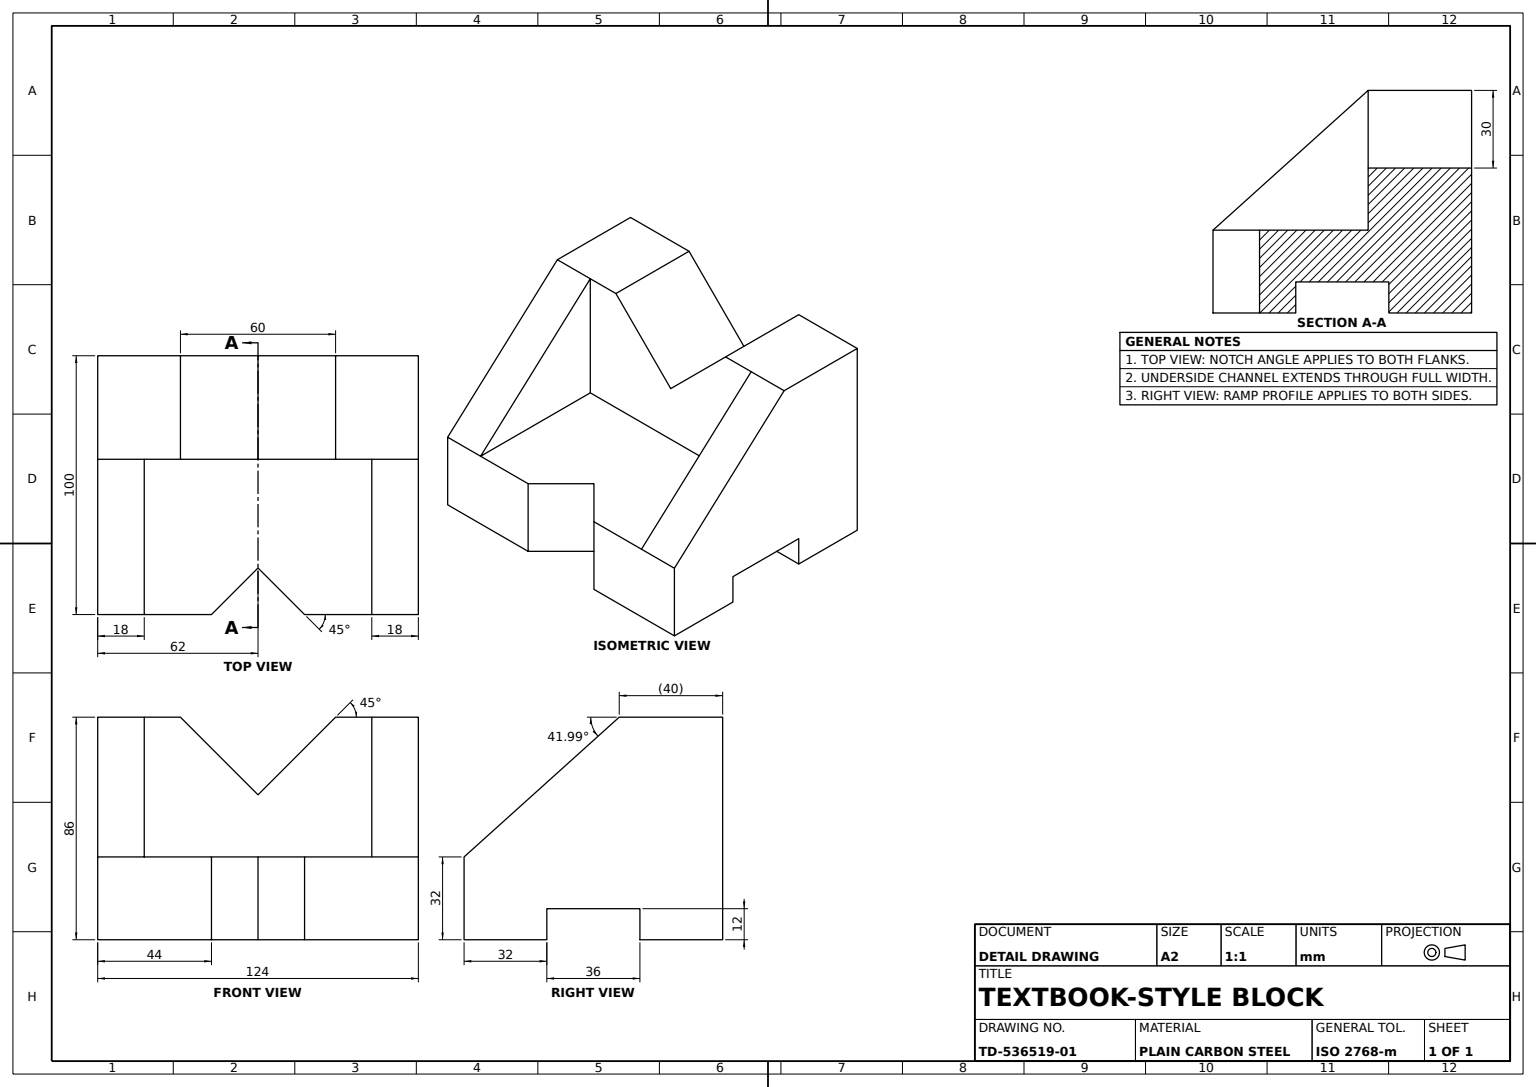
SolidWorks part; units mm, degrees
material "Plain Carbon Steel"
ref_plane "Front Plane" through (0, 0, 0) normal (0, 0, 1) x (1, 0, 0)
ref_plane "Top Plane" through (0, 0, 0) normal (0, 1, 0) x (1, 0, 0)
ref_plane "Right Plane" through (0, 0, 0) normal (1, 0, 0) x (0, 0, -1)
sketch "V-Block Profile Sketch" plane through (0, 0, 0) normal (0, 0, 1) x (1, 0, 0)
  line L0 (-30, 43) -> (0, 13)
  line L1 (-62, -43) -> (62, -43)
  line L2 (-62, -43) -> (-62, 43)
  line L3 (-62, 43) -> (-30, 43)
  line L4 (62, -43) -> (62, 43)
  line L5 (-62, -43) -> (62, 43) construction
  line L6 (-62, 43) -> (62, -43) construction
  line L7 (0, 13) -> (30, 43)
  line L8 (30, 43) -> (62, 43)
  point P0 (0, 0)
  dimension "D1" = 124
  dimension "24" = 86
  dimension "D2" = 60
  dimension "D3" = 32
  dimension "D4" = 30
extrude "V-Block Body 100" add sketch "V-Block Profile Sketch" along normal blind 100
sketch "Central Channel Sketch" plane through (-62, 0, 0) normal (-1, 0, 0) x (0, 0, 1)
  line L0 (100, -43) -> (0, -43) construction
  line L1 (32, -43) -> (68, -43)
  line L2 (32, -43) -> (32, -31)
  line L3 (32, -31) -> (68, -31)
  line L4 (68, -43) -> (68, -31)
  line L5 (100, 43) -> (100, -43) construction
  line L6 (40, 43) -> (100, -11)
  line L8 (100, 43) -> (0, 43) construction
  line L9 (0, 43) -> (0, -43) construction
  line L10 (40, 43) -> (100, 43)
  line L11 (100, 43) -> (100, -11)
  dimension "D1" = 12
  dimension "D2" = 36
  dimension "D3" = 32
  dimension "D4" = 40
  dimension "D5" = 32
extrude "Central Channel Cut" cut sketch "Central Channel Sketch" against normal through all
sketch "Square Pocket Sketch" plane through (0, -43, 0) normal (0, -1, 0) x (1, 0, 0)
  line L0 (62, 100) -> (-62, 100) construction
  line L1 (-44, 100) -> (44, 100)
  line L2 (-44, 100) -> (-44, 40)
  line L3 (-44, 40) -> (44, 40)
  line L4 (44, 100) -> (44, 40)
  line L5 (62, 40) -> (62, 100) construction
  line L6 (-62, 40) -> (-62, 100) construction
  line L7 (62, 40) -> (30, 40) construction
  dimension "D1" = 18
  dimension "D2" = 18
extrude "Square Pocket 18x18" cut sketch "Square Pocket Sketch" against normal up to surface (54 mm away) from offset 32 up to face at (-46, 43, 20) offset against normal yes
sketch "Angled Notch Sketch" plane through (0, -11, 0) normal (0, 1, 0) x (1, 0, 0)
  line L0 (-18, -100) -> (0, -82)
  line L1 (44, -100) -> (-44, -100) construction
  line L2 (0, -82) -> (18, -100)
  line L3 (18, -100) -> (-18, -100)
  line L4 (44, -40) -> (44, -100) construction
  line L5 (0, -100) -> (0, -91.7473) construction
  dimension "D1" = 18
  dimension "D2" = 44
  dimension "D3" = 36
extrude "Angled Notch Cut" cut sketch "Angled Notch Sketch" against normal up to next
